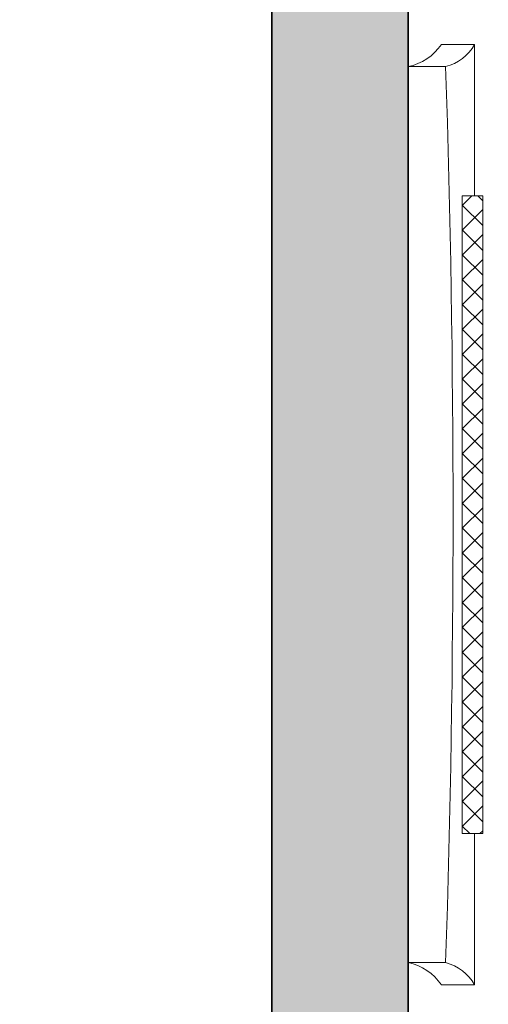
# Model space of a CAD drawing. Units: inches. Extents: x 2083 to 3317, y 1141 to 2115.
# Tile 4 of 256: x 2210 to 2241, y 1296 to 1361. Entities that reach past the tile are written whole.
import ezdxf

# ---------------------------------------------------------------- set-up
doc = ezdxf.new("R2010")
doc.units = ezdxf.units.IN
for name, color, linetype, lineweight in [('A-ANNO-DIMS', 2, 'Continuous', 18), ('A-FURN', 8, 'Continuous', 18), ('A-WALL', 7, 'Continuous', 35), ('www.cadblocksfree.com', 7, 'Continuous', 9)]:
    doc.layers.add(name, color=color, linetype=linetype, lineweight=lineweight)
doc.layers.add('A-WALL-PATT', color=251, linetype='Continuous', lineweight=13, true_color=0x636466)
doc.styles.get("Standard").update_dxf_attribs({"font": 'arial.ttf'})
doc.dimstyles.new('ISO-25', dxfattribs={"dimtxt": 12, "dimasz": 12, "dimexe": 1.25, "dimexo": 0.625, "dimtad": 1, "dimlunit": 3, "dimtxsty": 'Standard', "dimcen": 2.5, "dimadec": 0, "dimazin": 0, "dimtfac": 1, "dimtmove": 0, "dimatfit": 3, "dimfxl": 1, "dimarcsym": 0})

# ---------------------------------------------------------------- blocks, each defined once
blk = doc.blocks.new('bed')
at = {"layer": 'www.cadblocksfree.com', "ltscale": 0.2}
h = blk.add_hatch(dxfattribs=at)
h.set_pattern_fill('ANSI37,_O', color=256, scale=0.393701)
h.set_pattern_definition([(45, (2420.7222, -262.9689), (-0.8838835, 0.8838835), []), (135, (2420.7222, -262.9689), (-0.8838835, -0.8838835), [])])
h.paths.add_polyline_path([(3417.573, 1472.402), (3372.192, 1472.402), (3372.192, 1470.941), (3417.573, 1470.941)])
for p, q in [((3363.002, 1473.586), (3363.002, 1476.249)), ((3426.763, 1473.586), (3426.763, 1476.249)), ((3372.192, 1472.402), (3417.573, 1472.402)), ((3372.192, 1470.941), (3372.192, 1472.402)), ((3417.573, 1470.941), (3417.573, 1472.402)), ((3372.192, 1470.941), (3417.573, 1470.941))]:
    blk.add_line(p, q, dxfattribs=at)
for points in [[(3426.763, 1476.249), (3363.002, 1476.249)], [(3361.418, 1473.886), (3361.418, 1471.524), (3372.192, 1471.524)], [(3417.573, 1471.524), (3428.347, 1471.524), (3428.347, 1473.886)]]:
    blk.add_lwpolyline(points, dxfattribs=at)
for centre, radius, start, end in [((3359.334, 1476.997), 3.744, 303.82711, 348.4775), ((3430.432, 1476.997), 3.744, 191.5225, 236.17289), ((3359.844, 1474.373), 3.255, 298.91758, 345.9939), ((3394.883, 2431.358), 958.303, 268.093559, 271.906441), ((3429.921, 1474.373), 3.255, 194.0061, 241.08242)]:
    blk.add_arc(centre, radius, start, end, dxfattribs=at)
blk = doc.blocks.new('*D13')
at = {"layer": 'A-ANNO-DIMS', "color": 0, "lineweight": -2, "transparency": 16777216}
for p, q in [((2226.335, 1477.761), (2191.976, 1477.761)), ((2193.226, 1465.761), (2193.226, 1275.261)), ((2226.335, 1263.261), (2191.976, 1263.261))]:
    blk.add_line(p, q, dxfattribs=at)
at = {"layer": 'A-ANNO-DIMS', "color": 0, "transparency": 16777216}
for points in [[(2191.226, 1465.761), (2195.226, 1465.761), (2193.226, 1477.761)], [(2191.226, 1275.261), (2195.226, 1275.261), (2193.226, 1263.261)]]:
    blk.add_solid(points, dxfattribs=at)
at = {"layer": 'Defpoints', "color": 0, "transparency": 16777216}
for p in [(2226.96, 1477.761), (2193.226, 1263.261), (2226.96, 1263.261)]:
    blk.add_point(p, dxfattribs=at)
at = {"layer": 'A-ANNO-DIMS', "color": 0, "transparency": 16777216, "insert": (2186.474, 1370.511), "char_height": 12, "attachment_point": 5, "rotation": 90}
blk.add_mtext('17\'-10.5"', dxfattribs=at)
blk = doc.blocks.new('*D22')
at = {"layer": 'A-ANNO-DIMS', "color": 0, "lineweight": -2, "transparency": 16777216}
for p, q in [((2235.96, 1362.739), (2235.96, 1376.309)), ((2322.26, 1362.739), (2322.26, 1376.309)), ((2235.96, 1375.059), (2083.007, 1375.059)), ((2310.26, 1375.059), (2247.96, 1375.059))]:
    blk.add_line(p, q, dxfattribs=at)
at = {"layer": 'A-ANNO-DIMS', "color": 0, "transparency": 16777216}
for points in [[(2247.96, 1377.059), (2247.96, 1373.059), (2235.96, 1375.059)], [(2310.26, 1377.059), (2310.26, 1373.059), (2322.26, 1375.059)]]:
    blk.add_solid(points, dxfattribs=at)
at = {"layer": 'Defpoints', "color": 0, "transparency": 16777216}
for p in [(2235.96, 1375.059), (2235.96, 1362.114), (2322.26, 1362.114)]:
    blk.add_point(p, dxfattribs=at)
at = {"layer": 'A-ANNO-DIMS', "color": 0, "transparency": 16777216, "insert": (2153.483, 1381.889), "char_height": 12, "attachment_point": 5}
blk.add_mtext('BED 7\'-2 1/2" TYP.', dxfattribs=at)
blk = doc.blocks.new('*D47')
at = {"layer": 'A-ANNO-DIMS', "color": 0, "lineweight": -2, "transparency": 16777216}
for p, q in [((2235.335, 1416.261), (2173.36, 1416.261)), ((2174.61, 1284.261), (2174.61, 1404.261)), ((2235.335, 1272.261), (2173.36, 1272.261))]:
    blk.add_line(p, q, dxfattribs=at)
at = {"layer": 'A-ANNO-DIMS', "color": 0, "transparency": 16777216}
for points in [[(2172.61, 1404.261), (2176.61, 1404.261), (2174.61, 1416.261)], [(2172.61, 1284.261), (2176.61, 1284.261), (2174.61, 1272.261)]]:
    blk.add_solid(points, dxfattribs=at)
at = {"layer": 'Defpoints', "color": 0, "transparency": 16777216}
for p in [(2174.61, 1416.261), (2235.96, 1416.261), (2235.96, 1272.261)]:
    blk.add_point(p, dxfattribs=at)
at = {"layer": 'A-ANNO-DIMS', "color": 0, "transparency": 16777216, "insert": (2167.858, 1344.261), "char_height": 12, "attachment_point": 5, "rotation": 90}
blk.add_mtext('12\'-0"', dxfattribs=at)

msp = doc.modelspace()

# ---------------------------------------------------------------- hatches: boundary and pattern name
at = {"layer": 'A-WALL-PATT'}
h = msp.add_hatch(color=256, dxfattribs=at)
h.dxf.hatch_style = 1
h.paths.add_polyline_path([(3126.96, 2020.761), (2748.96, 2020.761), (2604.96, 2020.761), (2226.96, 2020.761), (2226.96, 1702.761), (2466.96, 1702.761), (2466.96, 1582.761), (2418.96, 1582.761), (2418.96, 1477.761), (2226.96, 1477.761), (2226.96, 1263.261), (2544.96, 1263.261), (2544.96, 1411.761), (2604.96, 1411.761), (2685.96, 1411.761), (2685.96, 1420.761), (2604.96, 1420.761), (2604.96, 1573.761), (2604.96, 1702.761), (2604.96, 2011.761), (2748.96, 2011.761), (2748.96, 1702.761), (2862.96, 1702.761), (2862.96, 1621.761), (2871.96, 1621.761), (2871.96, 1702.761), (2883.96, 1702.761), (2883.96, 1706.939, -0.026459), (2883.96, 1711.761), (2757.96, 1711.761), (2757.96, 1807.761), (2787.96, 1807.761), (2787.96, 1812.261), (2757.96, 1812.261), (2757.96, 2011.761), (2877.96, 2011.761), (2877.96, 1812.261), (2847.96, 1812.261), (2847.96, 1807.761), (2889.836, 1807.761), (2889.836, 1812.261), (2882.46, 1812.261), (2882.46, 2011.761), (3117.96, 2011.761), (3117.96, 1812.261), (2937.836, 1812.261), (2937.836, 1807.761), (2995.71, 1807.761), (2995.71, 1796.118), (3000.21, 1796.118), (3000.21, 1807.761), (3117.96, 1807.761), (3117.96, 1711.761), (3000.21, 1711.761), (3000.21, 1760.118), (2998.573, 1760.118, -0.020711), (2995.71, 1760.118), (2995.71, 1711.761), (2931.96, 1711.761), (2931.96, 1702.761), (3126.96, 1702.761)])
h.paths.add_polyline_path([(2471.46, 2011.761), (2471.46, 1810.011), (2462.717, 1810.011), (2462.717, 1805.511), (2505.96, 1805.511), (2505.96, 1810.011), (2475.96, 1810.011), (2475.96, 2011.761), (2595.96, 2011.761), (2595.96, 1810.011), (2565.96, 1810.011), (2565.96, 1805.511), (2595.96, 1805.511), (2595.96, 1711.761), (2235.96, 1711.761), (2235.96, 1805.511), (2353.71, 1805.511), (2353.71, 1796.054), (2358.21, 1796.054), (2358.21, 1805.511), (2414.717, 1805.511), (2414.717, 1810.011), (2235.96, 1810.011), (2235.96, 2011.761)], flags=16)
h.paths.add_polyline_path([(2270.205, 1994.61), (2270.205, 1970.61), (2246.205, 1970.61), (2246.205, 1994.61)], flags=0)
edge = h.paths.add_edge_path(flags=0)
edge.add_ellipse((2332.027, 1899.798), major_axis=(-3.043, 3.043), ratio=0.168252, start_angle=-161.33217, end_angle=-156.30711, ccw=False)
edge.add_ellipse((2333.082, 1898.744), major_axis=(-1.055, 1.055), ratio=0.453532, start_angle=-123.37102, end_angle=-94.15911)
edge = h.paths.add_edge_path(flags=0)
edge.add_ellipse((2332.027, 1968.876), major_axis=(3.043, 3.043), ratio=0.168252, start_angle=18.66783, end_angle=23.69289)
edge.add_spline(control_points=[(2332.926, 1970.691), (2332.227, 1970.336), (2330.894, 1969.659), (2328.413, 1970.932), (2327.204, 1967.749), (2324.71, 1969.956), (2322.533, 1967.012), (2320.013, 1971.296), (2317.68, 1968.158), (2316.041, 1967.102), (2315.427, 1966.81)], knot_values=[0, 0, 0, 0, 2.267059, 4.324559, 6.685584, 8.878641, 11.121502, 14.300359, 17.755284, 19.732645, 19.732645, 19.732645, 19.732645], degree=3, periodic=0)
edge.add_ellipse((2332.027, 1968.876), major_axis=(3.043, 3.043), ratio=0.168252, start_angle=18.66783, end_angle=23.69289, ccw=False)
edge.add_ellipse((2333.082, 1969.931), major_axis=(1.055, 1.055), ratio=0.453532, start_angle=56.62898, end_angle=85.84089, ccw=False)
edge = h.paths.add_edge_path(flags=0)
edge.add_spline(control_points=[(2296.428, 1967.988), (2293.628, 1965.336), (2287.704, 1959.727), (2299.744, 1949.996), (2294.533, 1935.669), (2290.573, 1920.604), (2293.394, 1909.974), (2296.185, 1904.967)], knot_values=[0.099185, 0.099185, 0.099185, 0.099185, 0.345301, 0.619822, 0.982653, 1.386093, 1.810555, 1.810555, 1.810555, 1.810555], degree=3, periodic=0)
edge.add_spline(control_points=[(2296.185, 1904.967), (2297.384, 1902.619), (2298.001, 1901.949), (2298.553, 1901.468)], knot_values=[0.006246, 0.006246, 0.006246, 0.006246, 0.055476, 0.055476, 0.055476, 0.055476], degree=3, periodic=0)
edge.add_spline(control_points=[(2298.553, 1901.468), (2297.259, 1900.923), (2295.225, 1900.232), (2293.06, 1900.614), (2292.101, 1900.788), (2292.09, 1900.791)], knot_values=[0.312835, 0.312835, 0.312835, 0.312835, 0.40178, 0.474987, 0.475903, 0.475903, 0.475903, 0.475903], degree=3, periodic=0)
edge.add_arc((2292.794, 1904.664), 3.937, 215.4209, 259.69818, ccw=False)
edge.add_spline(control_points=[(2289.585, 1902.382), (2289.477, 1902.535), (2289.368, 1902.688), (2289.261, 1902.841)], knot_values=[0.102872, 0.102872, 0.102872, 0.102872, 0.116896, 0.116896, 0.116896, 0.116896], degree=3, periodic=0)
edge.add_spline(control_points=[(2289.261, 1902.841), (2288.687, 1902.55), (2287.64, 1902.02), (2285.881, 1901.874), (2283.853, 1901.504), (2281.72, 1899.711), (2278.467, 1899.493), (2276.157, 1901.883), (2272.259, 1899.804), (2267.778, 1901.843), (2262.244, 1900.184), (2257.415, 1901.782), (2254.318, 1900.726), (2253.178, 1900.337)], knot_values=[0, 0, 0, 0, 1.907977, 3.477176, 5.261074, 7.972851, 11.680248, 13.717921, 16.939592, 22.789562, 27.502503, 33.595215, 37.145618, 37.145618, 37.145618, 37.145618], degree=3, periodic=0)
edge.add_line((2253.178, 1900.337), (2250.244, 1902.841))
edge.add_line((2250.244, 1902.841), (2250.244, 1965.833))
edge.add_line((2250.244, 1965.833), (2253.178, 1968.337))
edge.add_spline(control_points=[(2253.178, 1968.337), (2254.318, 1967.948), (2257.415, 1966.892), (2262.244, 1968.49), (2267.778, 1966.831), (2271.527, 1968.537), (2273.876, 1967.828), (2274.207, 1967.728)], knot_values=[0, 0, 0, 0, 0.09018, 0.244935, 0.364644, 0.513233, 0.537855, 0.537855, 0.537855, 0.537855], degree=3, periodic=0)
edge.add_arc((2274.353, 1963.793), 3.937, 72.05113, 92.12795, ccw=False)
edge.add_arc((2281.297, 1985.23), 18.596, 252.05113, 288.56572)
edge.add_arc((2292.317, 1956.029), 12.646, 71.02679, 113.77822, ccw=False)
edge = h.paths.add_edge_path(flags=0)
edge.add_spline(control_points=[(2274.899, 1951.856), (2275.066, 1951.617), (2275.233, 1951.377), (2275.398, 1951.136)], knot_values=[1.409916, 1.409916, 1.409916, 1.409916, 1.43159, 1.43159, 1.43159, 1.43159], degree=3, periodic=0)
edge.add_spline(control_points=[(2275.398, 1951.136), (2275.792, 1950.562), (2276.179, 1949.984), (2276.546, 1949.397)], knot_values=[1.358238, 1.358238, 1.358238, 1.358238, 1.409916, 1.409916, 1.409916, 1.409916], degree=3, periodic=0)
edge.add_line((2276.546, 1949.397), (2277.437, 1947.862))
edge.add_spline(control_points=[(2277.437, 1947.862), (2276.304, 1945.673), (2274.64, 1942.427), (2274.632, 1938.094), (2272.799, 1930.852), (2274.356, 1943.897), (2275.948, 1947.923), (2276.546, 1949.397)], knot_values=[0.005632, 0.005632, 0.005632, 0.005632, 0.186014, 0.266002, 0.357087, 0.59639, 0.739732, 0.739732, 0.739732, 0.739732], degree=3, periodic=0)
edge.add_spline(control_points=[(2276.546, 1949.397), (2276.179, 1949.984), (2275.792, 1950.562), (2275.398, 1951.136)], knot_values=[1.358238, 1.358238, 1.358238, 1.358238, 1.409916, 1.409916, 1.409916, 1.409916], degree=3, periodic=0)
edge.add_spline(control_points=[(2275.398, 1951.136), (2274.943, 1950.08), (2274.208, 1948.025), (2273.935, 1944.851), (2272.469, 1937.627), (2273.466, 1945.696), (2274.701, 1951.059), (2274.899, 1951.856)], knot_values=[0.104364, 0.104364, 0.104364, 0.104364, 0.189636, 0.269624, 0.36071, 0.600013, 0.644622, 0.644622, 0.644622, 0.644622], degree=3, periodic=0)
h.paths.add_polyline_path([(2269.168, 1963.128, -0.357527), (2268.171, 1960.976, -0.092561), (2268.171, 1939.436, -0.357527), (2269.168, 1937.285, -0.357527), (2267.016, 1938.282, -0.164785), (2254.686, 1938.282, -0.357527), (2252.534, 1937.285, -0.357527), (2253.531, 1939.436, -0.092561), (2253.531, 1960.976, -0.357527), (2252.534, 1963.128, -0.357527), (2254.686, 1962.131, -0.164785), (2267.016, 1962.131, -0.357527)], flags=0)
h.paths.add_polyline_path([(2248.874, 1967.802), (2248.874, 1957.028), (2249.458, 1957.028), (2249.458, 1911.647), (2248.874, 1911.647), (2248.874, 1900.873), (2246.512, 1900.873, 0.197327), (2244.15, 1902.457), (2244.15, 1966.218, 0.197327), (2246.512, 1967.802)], flags=0)
h.paths.add_polyline_path([(2269.168, 1931.389, -0.357527), (2268.171, 1929.238, -0.092561), (2268.171, 1907.698, -0.357527), (2269.168, 1905.547, -0.357527), (2267.016, 1906.544, -0.164785), (2254.686, 1906.544, -0.357527), (2252.534, 1905.547, -0.357527), (2253.531, 1907.698, -0.092561), (2253.531, 1929.238, -0.357527), (2252.534, 1931.389, -0.357527), (2254.686, 1930.392, -0.164785), (2267.016, 1930.392, -0.357527)], flags=0)
edge = h.paths.add_edge_path(flags=0)
edge.add_spline(control_points=[(2276.197, 1906.724), (2276.168, 1909.029), (2276.114, 1913.372), (2270.598, 1924.925), (2273.905, 1919.013), (2275.922, 1916.262), (2275.475, 1912.402), (2277.258, 1910.381), (2276.696, 1908.225), (2276.646, 1906.813), (2276.618, 1906.008)], knot_values=[0, 0, 0, 0, 8.61026, 16.221274, 18.843057, 23.804898, 27.440828, 29.356102, 31.203478, 33.650687, 33.650687, 33.650687, 33.650687], degree=3, periodic=0)
edge.add_spline(control_points=[(2276.618, 1906.008), (2276.623, 1905.624), (2276.498, 1904.629), (2275.442, 1903.855), (2274.937, 1903.08), (2274.859, 1902.841)], knot_values=[0.156488, 0.156488, 0.156488, 0.156488, 0.184398, 0.231376, 0.250598, 0.250598, 0.250598, 0.250598], degree=3, periodic=0)
edge.add_line((2274.859, 1902.841), (2276.506, 1902.841))
edge.add_spline(control_points=[(2276.506, 1902.841), (2276.788, 1903.085), (2277.665, 1904.125), (2278.25, 1904.341), (2277.654, 1908.527), (2278.156, 1906.228), (2278.1, 1905.286), (2278.847, 1904.069), (2277.857, 1903.415), (2277.874, 1902.991), (2277.904, 1902.841)], knot_values=[0.059574, 0.059574, 0.059574, 0.059574, 0.080753, 0.103741, 0.16972, 0.176036, 0.207137, 0.240474, 0.262341, 0.27366, 0.27366, 0.27366, 0.27366], degree=3, periodic=0)
edge.add_line((2277.904, 1902.841), (2280.03, 1902.841))
edge.add_spline(control_points=[(2280.03, 1902.841), (2279.888, 1903.088), (2279.499, 1903.982), (2280.152, 1905.939), (2278.104, 1909.658), (2279.762, 1907.185), (2280.328, 1904.875), (2280.485, 1903.49), (2281.463, 1903.249), (2281.758, 1902.936), (2281.834, 1902.841)], knot_values=[0.013856, 0.013856, 0.013856, 0.013856, 0.034874, 0.088867, 0.107879, 0.126738, 0.158714, 0.193757, 0.217487, 0.226722, 0.226722, 0.226722, 0.226722], degree=3, periodic=0)
edge.add_spline(control_points=[(2281.834, 1902.841), (2281.788, 1902.827), (2281.647, 1902.783), (2281.396, 1902.859), (2281.088, 1902.985), (2280.721, 1903.061), (2280.333, 1903.026), (2280.125, 1902.899), (2280.03, 1902.841)], knot_values=[0, 0, 0, 0, 0.14413, 0.435517, 0.749276, 1.153046, 1.548371, 1.878348, 1.878348, 1.878348, 1.878348], degree=3, periodic=0)
edge.add_line((2280.03, 1902.841), (2277.904, 1902.841))
edge.add_spline(control_points=[(2277.904, 1902.841), (2277.893, 1902.796), (2277.865, 1902.68), (2277.607, 1902.687), (2277.274, 1902.801), (2276.838, 1902.62), (2276.584, 1902.789), (2276.506, 1902.841)], knot_values=[0, 0, 0, 0, 0.127189, 0.326199, 0.628009, 1.24357, 1.515331, 1.515331, 1.515331, 1.515331], degree=3, periodic=0)
edge.add_line((2276.506, 1902.841), (2274.859, 1902.841))
edge.add_spline(control_points=[(2274.859, 1902.841), (2274.814, 1902.899), (2274.725, 1903.013), (2274.493, 1903.119), (2274.244, 1902.961), (2273.937, 1903.185), (2273.614, 1902.983), (2273.408, 1902.883), (2273.322, 1902.841)], knot_values=[0, 0, 0, 0, 0.21843, 0.436957, 0.687977, 0.990379, 1.398396, 1.69185, 1.69185, 1.69185, 1.69185], degree=3, periodic=0)
edge.add_spline(control_points=[(2273.322, 1902.841), (2273.617, 1903.446), (2274.274, 1904.538), (2276.027, 1904.574), (2276.207, 1906.584), (2276.197, 1906.724)], knot_values=[0.012227, 0.012227, 0.012227, 0.012227, 0.059472, 0.106218, 0.134458, 0.134458, 0.134458, 0.134458], degree=3, periodic=0)
h.paths.add_polyline_path([(2270.776, 1897.79), (2270.776, 1873.79), (2246.776, 1873.79), (2246.776, 1897.79)], flags=0)
h.paths.add_polyline_path([(2353.71, 1760.005), (2353.71, 1760.054), (2358.21, 1760.054, -0.033729)], flags=0)
h.paths.add_polyline_path([(2321.819, 1737.529), (2341.995, 1737.529, -0.414214), (2343.203, 1736.321), (2343.203, 1721.021, -0.414214), (2341.995, 1719.813), (2321.819, 1719.813, -0.414214), (2320.611, 1721.021), (2320.611, 1736.321, -0.414214)], flags=0)
h.paths.add_polyline_path([(2324.235, 1736.321), (2339.579, 1736.321, -0.414214), (2341.995, 1733.905), (2341.995, 1725.45, -0.414214), (2339.579, 1723.034), (2333.681, 1723.034), (2333.845, 1722.045, -0.870646), (2335.425, 1721.826, -0.767327), (2333.923, 1721.423), (2331.291, 1721.423, -0.767327), (2329.788, 1721.826, -0.870646), (2331.368, 1722.045), (2331.533, 1723.034), (2324.235, 1723.034, -0.414214), (2321.819, 1725.45), (2321.819, 1733.905, -0.414214)], flags=0)
h.paths.add_polyline_path([(2570.484, 1928.615), (2589.684, 1928.615), (2590.169, 1928.615), (2590.169, 1904.993), (2570.484, 1904.993)], flags=0)
h.paths.add_polyline_path([(2574.447, 1927.264, -1), (2572.829, 1927.264, -1)], flags=0)
h.paths.add_polyline_path([(2573.09, 1926.941), (2573.925, 1927.776), (2574.148, 1927.553), (2573.313, 1926.718)], flags=0)
h.paths.add_polyline_path([(2578.779, 1919.73, -1), (2571.592, 1919.73, -1)], flags=0)
h.paths.add_polyline_path([(2578.385, 1919.73, -1), (2571.985, 1919.73, -1)], flags=0)
h.paths.add_polyline_path([(2331.596, 1729.476, -1), (2333.618, 1729.476, -1)], flags=0)
h.paths.add_polyline_path([(2578.034, 1927.264, -1), (2576.416, 1927.264, -1)], flags=0)
h.paths.add_polyline_path([(2576.689, 1927.531), (2576.912, 1927.754), (2577.747, 1926.919), (2577.524, 1926.696)], flags=0)
h.paths.add_polyline_path([(2578.139, 1909.86, -1), (2572.232, 1909.86, -1)], flags=0)
h.paths.add_polyline_path([(2577.745, 1909.86, -1), (2572.625, 1909.86, -1)], flags=0)
h.paths.add_polyline_path([(2583.798, 1927.264, -1), (2582.179, 1927.264, -1)], flags=0)
h.paths.add_polyline_path([(2582.719, 1927.754), (2583.554, 1926.919), (2583.331, 1926.696), (2582.496, 1927.531)], flags=0)
h.paths.add_polyline_path([(2582.496, 1927.531), (2582.719, 1927.754), (2583.554, 1926.919), (2583.331, 1926.696)], flags=0)
h.paths.add_polyline_path([(2587.739, 1920.53, -1), (2581.832, 1920.53, -1)], flags=0)
h.paths.add_polyline_path([(2587.345, 1920.53, -1), (2582.225, 1920.53, -1)], flags=0)
h.paths.add_polyline_path([(2587.385, 1927.264, -1), (2585.766, 1927.264, -1)], flags=0)
h.paths.add_polyline_path([(2586.082, 1926.98), (2586.917, 1927.815), (2587.14, 1927.593), (2586.305, 1926.758)], flags=0)
h.paths.add_polyline_path([(2588.379, 1910.66, -1), (2581.192, 1910.66, -1)], flags=0)
h.paths.add_polyline_path([(2587.985, 1910.66, -1), (2581.585, 1910.66, -1)], flags=0)
h.paths.add_polyline_path([(2417.168, 1729.478), (2437.344, 1729.478, -0.414214), (2438.552, 1728.27), (2438.552, 1712.969, -0.414214), (2437.344, 1711.761), (2417.168, 1711.761, -0.414214), (2415.96, 1712.969), (2415.96, 1728.27, -0.414214)], flags=0)
h.paths.add_polyline_path([(2419.584, 1728.27), (2434.928, 1728.27, -0.414214), (2437.344, 1725.854), (2437.344, 1717.398, -0.414214), (2434.928, 1714.983), (2429.029, 1714.983), (2429.194, 1713.994, -0.870646), (2430.774, 1713.775, -0.767327), (2429.271, 1713.372), (2426.64, 1713.372, -0.767327), (2425.137, 1713.775, -0.870646), (2426.717, 1713.994), (2426.882, 1714.983), (2419.584, 1714.983, -0.414214), (2417.168, 1717.398), (2417.168, 1725.854, -0.414214)], flags=0)
h.paths.add_polyline_path([(2419.584, 1728.27), (2434.928, 1728.27, -0.414214), (2437.344, 1725.854), (2437.344, 1717.398, -0.414214), (2434.928, 1714.983), (2429.029, 1714.983), (2428.358, 1719.009), (2427.553, 1719.009), (2426.882, 1714.983), (2419.584, 1714.983, -0.414214), (2417.168, 1717.398), (2417.168, 1725.854, -0.414214)], flags=0)
h.paths.add_polyline_path([(2426.944, 1721.425, -1), (2428.967, 1721.425, -1)], flags=0)
h.paths.add_polyline_path([(2475.96, 1702.761), (2595.96, 1702.761), (2595.96, 1582.761), (2475.96, 1582.761)], flags=16)
h.paths.add_polyline_path([(2427.96, 1573.761), (2595.96, 1573.761), (2595.96, 1468.761), (2595.96, 1420.761), (2384.46, 1420.761), (2384.46, 1468.761), (2427.96, 1468.761)], flags=16)
h.paths.add_polyline_path([(2379.96, 1468.761), (2379.96, 1420.761), (2235.96, 1420.761), (2235.96, 1468.761)], flags=16)
h.paths.add_polyline_path([(2317.816, 1466.696), (2337.992, 1466.696, -0.414214), (2339.2, 1465.488), (2339.2, 1450.187, -0.414214), (2337.992, 1448.979), (2317.816, 1448.979, -0.414214), (2316.608, 1450.187), (2316.608, 1465.488, -0.414214)], flags=0)
h.paths.add_polyline_path([(2320.232, 1465.488), (2335.576, 1465.488, -0.414214), (2337.992, 1463.072), (2337.992, 1454.616, -0.414214), (2335.576, 1452.2), (2329.677, 1452.2), (2329.842, 1451.212, -0.870646), (2331.422, 1450.992, -0.767327), (2329.92, 1450.59), (2327.288, 1450.59, -0.767327), (2325.785, 1450.992, -0.870646), (2327.365, 1451.212), (2327.53, 1452.2), (2320.232, 1452.2, -0.414214), (2317.816, 1454.616), (2317.816, 1463.072, -0.414214)], flags=0)
h.paths.add_polyline_path([(2320.232, 1465.488), (2335.576, 1465.488, -0.414214), (2337.992, 1463.072), (2337.992, 1454.616, -0.414214), (2335.576, 1452.2), (2329.677, 1452.2), (2329.006, 1456.227), (2328.201, 1456.227), (2327.53, 1452.2), (2320.232, 1452.2, -0.414214), (2317.816, 1454.616), (2317.816, 1463.072, -0.414214)], flags=0)
h.paths.add_polyline_path([(2327.593, 1458.643, -1), (2329.615, 1458.643, -1)], flags=0)
h.paths.add_polyline_path([(2244.412, 1433.34), (2241.921, 1433.34, -0.414214), (2240.018, 1435.244), (2240.018, 1440.953, -0.414211), (2241.921, 1442.856), (2244.412, 1442.856, -1.976472)], flags=0)
h.paths.add_polyline_path([(2245.357, 1434.398, -0.414214), (2245.357, 1441.799, -2.144098)], flags=0)
h.paths.add_polyline_path([(2535.96, 1416.261), (2535.96, 1272.261), (2235.96, 1272.261), (2235.96, 1416.261)], flags=16)
h.paths.add_polyline_path([(2260.12, 1384.293), (2260.12, 1362.039), (2237.865, 1362.039), (2237.865, 1384.293)], flags=0)
edge = h.paths.add_edge_path(flags=0)
edge.add_line((2318.252, 1362.093), (2318.146, 1362.001))
edge.add_ellipse((2317.445, 1360.431), major_axis=(2.822, 2.822), ratio=0.168252, start_angle=18.66783, end_angle=20.94813, ccw=False)
edge.add_ellipse((2318.423, 1361.409), major_axis=(0.978, 0.978), ratio=0.453532, start_angle=56.62898, end_angle=70.2262, ccw=False)
edge = h.paths.add_edge_path(flags=0)
edge.add_line((2319.107, 1295.571), (2319.015, 1295.677))
edge.add_ellipse((2317.445, 1296.378), major_axis=(-2.822, 2.822), ratio=0.168252, start_angle=-161.33217, end_angle=-159.05187, ccw=False)
edge.add_ellipse((2318.423, 1295.4), major_axis=(-0.978, 0.978), ratio=0.453532, start_angle=-123.37102, end_angle=-109.7738)
edge = h.paths.add_edge_path(flags=0)
edge.add_spline(control_points=[(2284.21, 1301.17), (2284.581, 1300.445), (2284.891, 1299.892), (2285.16, 1299.461)], knot_values=[0.039066, 0.039066, 0.039066, 0.039066, 0.055476, 0.055476, 0.055476, 0.055476], degree=3, periodic=0)
edge.add_line((2285.16, 1299.461), (2284.21, 1301.17))
edge = h.paths.add_edge_path(flags=0)
edge.add_line((2280.412, 1297.298), (2283.37, 1297.036))
edge.add_line((2283.37, 1297.036), (2286.406, 1297.926))
edge.add_spline(control_points=[(2286.406, 1297.926), (2285.305, 1297.463), (2284.345, 1297.129), (2283.37, 1297.036)], knot_values=[0.394369, 0.394369, 0.394369, 0.394369, 0.475903, 0.475903, 0.475903, 0.475903], degree=3, periodic=0)
edge.add_spline(control_points=[(2283.37, 1297.036), (2283.281, 1297.028), (2282.316, 1296.957), (2281.313, 1297.134), (2280.423, 1297.296), (2280.412, 1297.298)], knot_values=[0.312835, 0.312835, 0.312835, 0.312835, 0.320246, 0.393453, 0.394369, 0.394369, 0.394369, 0.394369], degree=3, periodic=0)
edge = h.paths.add_edge_path(flags=0)
edge.add_line((2284.436, 1359.607), (2280.446, 1355.328))
edge.add_line((2280.446, 1355.328), (2279.58, 1351.018))
edge.add_line((2279.58, 1351.018), (2282.413, 1346.58))
edge.add_spline(control_points=[(2282.413, 1346.58), (2283.153, 1345.589), (2284.253, 1344.029), (2284.801, 1342.387), (2284.935, 1341.806)], knot_values=[1.240098, 1.240098, 1.240098, 1.240098, 1.332892, 1.382712, 1.382712, 1.382712, 1.382712], degree=3, periodic=0)
edge.add_spline(control_points=[(2284.935, 1341.806), (2285.319, 1340.141), (2285.233, 1338.409), (2284.91, 1336.654)], knot_values=[1.097484, 1.097484, 1.097484, 1.097484, 1.240098, 1.240098, 1.240098, 1.240098], degree=3, periodic=0)
edge.add_spline(control_points=[(2284.91, 1336.654), (2284.587, 1334.899), (2284.027, 1333.12), (2283.463, 1331.361)], knot_values=[0.95487, 0.95487, 0.95487, 0.95487, 1.097484, 1.097484, 1.097484, 1.097484], degree=3, periodic=0)
edge.add_line((2283.463, 1331.361), (2281.89, 1326.153))
edge.add_line((2281.89, 1326.153), (2280.756, 1321.056))
edge.add_line((2280.756, 1321.056), (2280.299, 1316.002))
edge.add_line((2280.299, 1316.002), (2280.716, 1310.95))
edge.add_line((2280.716, 1310.95), (2282.028, 1305.972))
edge.add_line((2282.028, 1305.972), (2284.21, 1301.17))
edge.add_spline(control_points=[(2284.21, 1301.17), (2283.341, 1302.73), (2282.612, 1304.336), (2282.028, 1305.972)], knot_values=[0.099185, 0.099185, 0.099185, 0.099185, 0.241799, 0.241799, 0.241799, 0.241799], degree=3, periodic=0)
edge.add_spline(control_points=[(2282.028, 1305.972), (2281.444, 1307.608), (2281.005, 1309.273), (2280.716, 1310.95)], knot_values=[0.241799, 0.241799, 0.241799, 0.241799, 0.384413, 0.384413, 0.384413, 0.384413], degree=3, periodic=0)
edge.add_spline(control_points=[(2280.716, 1310.95), (2280.433, 1312.588), (2280.289, 1314.277), (2280.299, 1315.962), (2280.299, 1316.002)], knot_values=[0.384413, 0.384413, 0.384413, 0.384413, 0.523647, 0.527028, 0.527028, 0.527028, 0.527028], degree=3, periodic=0)
edge.add_spline(control_points=[(2280.299, 1316.002), (2280.312, 1317.687), (2280.478, 1319.368), (2280.756, 1321.056)], knot_values=[0.527028, 0.527028, 0.527028, 0.527028, 0.669642, 0.669642, 0.669642, 0.669642], degree=3, periodic=0)
edge.add_spline(control_points=[(2280.756, 1321.056), (2281.035, 1322.744), (2281.426, 1324.44), (2281.89, 1326.153)], knot_values=[0.669642, 0.669642, 0.669642, 0.669642, 0.812256, 0.812256, 0.812256, 0.812256], degree=3, periodic=0)
edge.add_spline(control_points=[(2281.89, 1326.153), (2282.264, 1327.533), (2282.788, 1329.262), (2283.353, 1331.018), (2283.463, 1331.361)], knot_values=[0.812256, 0.812256, 0.812256, 0.812256, 0.927087, 0.95487, 0.95487, 0.95487, 0.95487], degree=3, periodic=0)
edge.add_line((2283.463, 1331.361), (2284.91, 1336.654))
edge.add_line((2284.91, 1336.654), (2284.935, 1341.806))
edge.add_line((2284.935, 1341.806), (2282.413, 1346.58))
edge.add_spline(control_points=[(2282.413, 1346.58), (2281.275, 1348.104), (2280.078, 1349.57), (2279.58, 1351.018)], knot_values=[1.382712, 1.382712, 1.382712, 1.382712, 1.525326, 1.525326, 1.525326, 1.525326], degree=3, periodic=0)
edge.add_spline(control_points=[(2279.58, 1351.018), (2279.443, 1351.415), (2279.136, 1352.857), (2279.735, 1354.29), (2280.446, 1355.328)], knot_values=[1.525326, 1.525326, 1.525326, 1.525326, 1.564439, 1.667941, 1.667941, 1.667941, 1.667941], degree=3, periodic=0)
edge.add_spline(control_points=[(2280.446, 1355.328), (2281.426, 1356.758), (2282.931, 1358.183), (2284.436, 1359.607)], knot_values=[1.667941, 1.667941, 1.667941, 1.667941, 1.810555, 1.810555, 1.810555, 1.810555], degree=3, periodic=0)
edge.add_arc((2280.623, 1348.518), 11.726, 71.02679, 113.77822)
edge.add_arc((2270.405, 1375.595), 17.244, 252.05113, 288.56572, ccw=False)
edge.add_arc((2263.966, 1355.718), 3.651, 72.05113, 92.12795)
edge.add_arc((2263.966, 1355.718), 3.651, 92.12795, 177.98513)
edge.add_spline(control_points=[(2260.318, 1355.846), (2260.26, 1354.221), (2260.551, 1350.187), (2262.999, 1346.766), (2264.473, 1344.649)], knot_values=[1.43159, 1.43159, 1.43159, 1.43159, 1.564144, 1.770695, 1.770695, 1.770695, 1.770695], degree=3, periodic=0)
edge.add_line((2264.473, 1344.649), (2264.936, 1343.983))
edge.add_spline(control_points=[(2263.801, 1340.248), (2263.843, 1340.514), (2264.067, 1341.756), (2264.513, 1343.002), (2264.935, 1343.981)], knot_values=[0.53657, 0.53657, 0.53657, 0.53657, 0.559349, 0.644622, 0.644622, 0.644622, 0.644622], degree=3, periodic=0)
edge.add_spline(control_points=[(2264.935, 1343.981), (2265.118, 1343.715), (2265.299, 1343.448), (2265.477, 1343.179)], knot_values=[1.384077, 1.384077, 1.384077, 1.384077, 1.409916, 1.409916, 1.409916, 1.409916], degree=3, periodic=0)
edge.add_spline(control_points=[(2265.477, 1343.179), (2265.655, 1342.911), (2265.829, 1342.641), (2265.999, 1342.369)], knot_values=[1.358238, 1.358238, 1.358238, 1.358238, 1.384077, 1.384077, 1.384077, 1.384077], degree=3, periodic=0)
edge.add_line((2265.999, 1342.369), (2266.826, 1340.946))
edge.add_spline(control_points=[(2266.826, 1340.946), (2268.894, 1337.09), (2271.398, 1325.843), (2270.516, 1310.569), (2275.919, 1301.861), (2277.79, 1299.199)], knot_values=[0.116896, 0.116896, 0.116896, 0.116896, 0.472987, 1.050969, 1.313793, 1.313793, 1.313793, 1.313793], degree=3, periodic=0)
edge.add_spline(control_points=[(2277.79, 1299.199), (2277.839, 1299.128), (2277.889, 1299.057), (2277.94, 1298.987)], knot_values=[0.109884, 0.109884, 0.109884, 0.109884, 0.116896, 0.116896, 0.116896, 0.116896], degree=3, periodic=0)
edge.add_line((2277.94, 1298.987), (2277.789, 1299.199))
edge.add_spline(control_points=[(2277.789, 1299.199), (2277.257, 1298.929), (2276.286, 1298.438), (2275.039, 1298.334), (2274.383, 1298.239), (2274.215, 1298.209)], knot_values=[33.12187, 33.12187, 33.12187, 33.12187, 35.029056, 36.598255, 37.144827, 37.144827, 37.144827, 37.144827], degree=3, periodic=0)
edge.add_line((2274.215, 1298.209), (2273.073, 1297.893))
edge.add_spline(control_points=[(2273.073, 1297.893), (2272.323, 1297.58), (2271.039, 1296.511), (2269.248, 1296.226), (2268.423, 1296.375)], knot_values=[26.532584, 26.532584, 26.532584, 26.532584, 29.198919, 31.839101, 31.839101, 31.839101, 31.839101], degree=3, periodic=0)
edge.add_line((2268.423, 1296.375), (2263.879, 1297.458))
edge.add_spline(control_points=[(2263.879, 1297.458), (2263.556, 1297.359), (2261.86, 1296.839), (2260.239, 1297.282), (2258.933, 1297.516)], knot_values=[15.919551, 15.919551, 15.919551, 15.919551, 16.939592, 21.226067, 21.226067, 21.226067, 21.226067], degree=3, periodic=0)
edge.add_line((2258.933, 1297.516), (2254.055, 1297.329))
edge.add_spline(control_points=[(2254.055, 1297.329), (2253.756, 1297.296), (2252.114, 1297.165), (2250.462, 1297.544), (2249.13, 1297.668)], knot_values=[5.306517, 5.306517, 5.306517, 5.306517, 6.276435, 10.613034, 10.613034, 10.613034, 10.613034], degree=3, periodic=0)
edge.add_line((2249.13, 1297.668), (2244.332, 1296.878))
edge.add_line((2244.332, 1296.878), (2241.611, 1299.199))
edge.add_line((2241.611, 1299.199), (2241.611, 1357.609))
edge.add_line((2241.611, 1357.609), (2244.332, 1359.931))
edge.add_line((2244.332, 1359.931), (2252.729, 1359.543))
edge.add_spline(control_points=[(2252.729, 1359.543), (2252.871, 1359.546), (2253.306, 1359.548), (2253.74, 1359.514), (2254.032, 1359.482)], knot_values=[0.233291, 0.233291, 0.233291, 0.233291, 0.244935, 0.268927, 0.268927, 0.268927, 0.268927], degree=3, periodic=0)
edge.add_line((2254.032, 1359.482), (2259.587, 1359.416))
edge.add_spline(control_points=[(2259.587, 1359.416), (2260.677, 1359.629), (2262.073, 1359.897), (2263.524, 1359.459), (2263.83, 1359.366)], knot_values=[0.422516, 0.422516, 0.422516, 0.422516, 0.513233, 0.537855, 0.537855, 0.537855, 0.537855], degree=3, periodic=0)
edge.add_arc((2263.966, 1355.718), 3.651, 72.05113, 92.12795, ccw=False)
edge.add_arc((2270.405, 1375.595), 17.244, 252.05113, 288.56572)
edge.add_arc((2280.623, 1348.518), 11.726, 71.02679, 113.77822, ccw=False)
h.paths.add_polyline_path([(2240.341, 1359.435), (2240.341, 1349.444), (2240.882, 1349.444), (2240.882, 1307.365), (2240.341, 1307.365), (2240.341, 1297.374), (2238.15, 1297.374, 0.197327), (2235.96, 1298.843), (2235.96, 1357.966, 0.197327), (2238.15, 1359.435)], flags=0)
h.paths.add_polyline_path([(2259.158, 1355.101, -0.357527), (2258.233, 1353.106, -0.092561), (2258.233, 1333.133, -0.357527), (2259.158, 1331.138, -0.357527), (2257.163, 1332.062, -0.164785), (2245.729, 1332.062, -0.357527), (2243.735, 1331.138, -0.357527), (2244.659, 1333.133, -0.092561), (2244.659, 1353.106, -0.357527), (2243.735, 1355.101, -0.357527), (2245.729, 1354.176, -0.164785), (2257.163, 1354.176, -0.357527)], flags=0)
edge = h.paths.add_edge_path(flags=0)
edge.add_line((2265.999, 1342.369), (2266.826, 1340.946))
edge.add_line((2266.826, 1340.946), (2265.308, 1337.814))
edge.add_line((2265.308, 1337.814), (2264.358, 1334.653))
edge.add_line((2264.358, 1334.653), (2264.262, 1333.8))
edge.add_spline(control_points=[(2264.262, 1333.8), (2264.208, 1333.187), (2264.162, 1332.366), (2264.007, 1331.414), (2263.969, 1331.202)], knot_values=[0.464444, 0.464444, 0.464444, 0.464444, 0.516691, 0.531608, 0.531608, 0.531608, 0.531608], degree=3, periodic=0)
edge.add_spline(control_points=[(2263.969, 1331.202), (2263.775, 1330.119), (2263.424, 1328.791), (2263.257, 1328.531), (2263.234, 1328.515)], knot_values=[0.372682, 0.372682, 0.372682, 0.372682, 0.44885, 0.464444, 0.464444, 0.464444, 0.464444], degree=3, periodic=0)
edge.add_spline(control_points=[(2263.234, 1328.515), (2263.096, 1328.42), (2263.131, 1329.301), (2263.275, 1330.616)], knot_values=[0.280919, 0.280919, 0.280919, 0.280919, 0.372682, 0.372682, 0.372682, 0.372682], degree=3, periodic=0)
edge.add_spline(control_points=[(2263.275, 1330.616), (2263.419, 1331.93), (2263.672, 1333.677), (2263.97, 1335.315)], knot_values=[0.189157, 0.189157, 0.189157, 0.189157, 0.280919, 0.280919, 0.280919, 0.280919], degree=3, periodic=0)
edge.add_spline(control_points=[(2263.97, 1335.315), (2264.1, 1336.032), (2264.419, 1337.622), (2264.755, 1338.864), (2264.947, 1339.491)], knot_values=[0.097394, 0.097394, 0.097394, 0.097394, 0.137578, 0.189157, 0.189157, 0.189157, 0.189157], degree=3, periodic=0)
edge.add_spline(control_points=[(2264.947, 1339.491), (2265.29, 1340.606), (2265.644, 1341.494), (2265.999, 1342.369)], knot_values=[0.005632, 0.005632, 0.005632, 0.005632, 0.097394, 0.097394, 0.097394, 0.097394], degree=3, periodic=0)
h.paths.add_polyline_path([(2259.158, 1325.671, -0.357527), (2258.233, 1323.676, -0.092561), (2258.233, 1303.703, -0.357527), (2259.158, 1301.708, -0.357527), (2257.163, 1302.633, -0.164785), (2245.729, 1302.633, -0.357527), (2243.735, 1301.708, -0.357527), (2244.659, 1303.703, -0.092561), (2244.659, 1323.676, -0.357527), (2243.735, 1325.671, -0.357527), (2245.729, 1324.747, -0.164785), (2257.163, 1324.747, -0.357527)], flags=0)
edge = h.paths.add_edge_path(flags=0)
edge.add_spline(control_points=[(2261.709, 1317.311), (2261.679, 1317.418), (2261.762, 1317.389), (2262.491, 1316.09), (2262.962, 1315.301)], knot_values=[14.955861, 14.955861, 14.955861, 14.955861, 16.221274, 18.694826, 18.694826, 18.694826, 18.694826], degree=3, periodic=0)
edge.add_spline(control_points=[(2262.962, 1315.301), (2262.99, 1315.254), (2263.702, 1314.067), (2264.349, 1313.127), (2264.73, 1312.164)], knot_values=[18.694826, 18.694826, 18.694826, 18.694826, 18.843057, 22.433791, 22.433791, 22.433791, 22.433791], degree=3, periodic=0)
edge.add_spline(control_points=[(2264.73, 1312.164), (2264.876, 1311.796), (2265.177, 1310.77), (2265.143, 1309.559), (2265.248, 1308.824)], knot_values=[22.433791, 22.433791, 22.433791, 22.433791, 23.804898, 26.172756, 26.172756, 26.172756, 26.172756], degree=3, periodic=0)
edge.add_line((2265.248, 1308.824), (2265.851, 1307.172))
edge.add_spline(control_points=[(2265.851, 1307.172), (2266.065, 1306.822), (2266.384, 1306.332), (2266.424, 1305.781), (2266.42, 1305.611)], knot_values=[28.062562, 28.062562, 28.062562, 28.062562, 29.356102, 29.911721, 29.911721, 29.911721, 29.911721], degree=3, periodic=0)
edge.add_spline(control_points=[(2266.42, 1305.611), (2266.416, 1305.433), (2266.394, 1305.25), (2266.365, 1305.066)], knot_values=[29.911721, 29.911721, 29.911721, 29.911721, 30.497837, 30.497837, 30.497837, 30.497837], degree=3, periodic=0)
edge.add_line((2266.365, 1305.066), (2266.066, 1302.136))
edge.add_spline(control_points=[(2266.066, 1302.136), (2266.071, 1301.78), (2265.998, 1301.2), (2265.663, 1300.759), (2265.509, 1300.586)], knot_values=[0.156488, 0.156488, 0.156488, 0.156488, 0.184398, 0.203543, 0.203543, 0.203543, 0.203543], degree=3, periodic=0)
edge.add_line((2265.509, 1300.586), (2264.435, 1299.199))
edge.add_line((2264.435, 1299.199), (2265.962, 1299.199))
edge.add_line((2265.962, 1299.199), (2267.336, 1301.175))
edge.add_line((2267.336, 1301.175), (2267.312, 1301.986))
edge.add_spline(control_points=[(2267.312, 1301.986), (2267.261, 1302.862), (2267.16, 1303.737), (2267.271, 1303.326)], knot_values=[0.126229, 0.126229, 0.126229, 0.126229, 0.166617, 0.166617, 0.166617, 0.166617], degree=3, periodic=0)
edge.add_spline(control_points=[(2267.271, 1303.326), (2267.28, 1303.294), (2267.31, 1303.175), (2267.373, 1302.884), (2267.406, 1302.683), (2267.418, 1302.601)], knot_values=[0.166617, 0.166617, 0.166617, 0.166617, 0.16972, 0.176036, 0.180765, 0.180765, 0.180765, 0.180765], degree=3, periodic=0)
edge.add_spline(control_points=[(2267.744, 1300.988), (2267.688, 1301.151), (2267.481, 1301.657), (2267.484, 1302.145), (2267.418, 1302.601)], knot_values=[0.180765, 0.180765, 0.180765, 0.180765, 0.193767, 0.220139, 0.220139, 0.220139, 0.220139], degree=3, periodic=0)
edge.add_line((2267.418, 1302.601), (2267.744, 1300.988))
edge.add_spline(control_points=[(2267.744, 1300.988), (2267.832, 1300.732), (2267.932, 1300.31), (2267.555, 1299.975), (2267.429, 1299.829)], knot_values=[0.220139, 0.220139, 0.220139, 0.220139, 0.240474, 0.25489, 0.25489, 0.25489, 0.25489], degree=3, periodic=0)
edge.add_line((2267.429, 1299.829), (2267.258, 1299.199))
edge.add_line((2267.258, 1299.199), (2269.23, 1299.199))
edge.add_spline(control_points=[(2269.23, 1299.199), (2269.099, 1299.429), (2268.843, 1300.016), (2269.012, 1300.916), (2268.947, 1301.661)], knot_values=[0.013856, 0.013856, 0.013856, 0.013856, 0.034874, 0.067073, 0.067073, 0.067073, 0.067073], degree=3, periodic=0)
edge.add_line((2268.947, 1301.661), (2268.432, 1303.603))
edge.add_spline(control_points=[(2268.432, 1303.603), (2268.176, 1304.192), (2267.596, 1305.251), (2268.041, 1304.623), (2268.251, 1304.282)], knot_values=[0.090155, 0.090155, 0.090155, 0.090155, 0.107879, 0.120289, 0.120289, 0.120289, 0.120289], degree=3, periodic=0)
edge.add_spline(control_points=[(2268.251, 1304.282), (2268.361, 1304.105), (2269.058, 1302.918), (2269.383, 1301.59), (2269.521, 1300.776), (2269.575, 1300.556)], knot_values=[0.120289, 0.120289, 0.120289, 0.120289, 0.126738, 0.158714, 0.173506, 0.173506, 0.173506, 0.173506], degree=3, periodic=0)
edge.add_line((2269.575, 1300.556), (2270.686, 1299.421))
edge.add_spline(control_points=[(2270.686, 1299.421), (2270.767, 1299.357), (2270.838, 1299.281), (2270.903, 1299.199)], knot_values=[0.21816, 0.21816, 0.21816, 0.21816, 0.226722, 0.226722, 0.226722, 0.226722], degree=3, periodic=0)
edge.add_line((2270.937, 1299.193), (2270.903, 1299.199))
edge.add_spline(control_points=[(2270.903, 1299.199), (2270.86, 1299.186), (2270.73, 1299.146), (2270.496, 1299.216), (2270.272, 1299.308), (2270.121, 1299.348), (2270.063, 1299.36)], knot_values=[0.939174, 0.939174, 0.939174, 0.939174, 1.083304, 1.374691, 1.68845, 1.878348, 1.878348, 1.878348, 1.878348], degree=3, periodic=0)
edge.add_line((2270.063, 1299.36), (2269.23, 1299.199))
edge.add_line((2269.23, 1299.199), (2267.258, 1299.199))
edge.add_spline(control_points=[(2267.258, 1299.199), (2267.248, 1299.157), (2267.223, 1299.05), (2266.984, 1299.057), (2266.809, 1299.116), (2266.677, 1299.109), (2266.637, 1299.105)], knot_values=[0.757665, 0.757665, 0.757665, 0.757665, 0.884854, 1.083864, 1.385675, 1.515331, 1.515331, 1.515331, 1.515331], degree=3, periodic=0)
edge.add_spline(control_points=[(2266.637, 1299.105), (2266.485, 1299.089), (2266.236, 1299.017), (2266.035, 1299.151), (2265.962, 1299.199)], knot_values=[0, 0, 0, 0, 0.485905, 0.757665, 0.757665, 0.757665, 0.757665], degree=3, periodic=0)
edge.add_line((2265.962, 1299.199), (2264.435, 1299.199))
edge.add_line((2264.435, 1299.199), (2263.858, 1299.367))
edge.add_spline(control_points=[(2263.858, 1299.367), (2263.819, 1299.371), (2263.78, 1299.386), (2263.74, 1299.402)], knot_values=[0.845925, 0.845925, 0.845925, 0.845925, 0.978627, 0.978627, 0.978627, 0.978627], degree=3, periodic=0)
edge.add_line((2263.722, 1299.396), (2263.01, 1299.199))
edge.add_spline(control_points=[(2263.01, 1299.199), (2263.246, 1299.683), (2263.506, 1300.128), (2263.873, 1300.408)], knot_values=[0.012227, 0.012227, 0.012227, 0.012227, 0.052971, 0.052971, 0.052971, 0.052971], degree=3, periodic=0)
edge.add_spline(control_points=[(2263.873, 1300.408), (2263.932, 1300.453), (2264.084, 1300.553), (2264.255, 1300.624), (2264.36, 1300.665)], knot_values=[0.052971, 0.052971, 0.052971, 0.052971, 0.059472, 0.069086, 0.069086, 0.069086, 0.069086], degree=3, periodic=0)
edge.add_line((2264.36, 1300.665), (2265.142, 1301.078))
edge.add_line((2265.142, 1301.078), (2265.676, 1302.8))
edge.add_line((2265.676, 1302.8), (2265.541, 1305.704))
edge.add_line((2265.541, 1305.704), (2264.803, 1309.328))
edge.add_line((2264.803, 1309.328), (2263.041, 1314.092))
edge.add_spline(control_points=[(2263.041, 1314.092), (2262.384, 1315.671), (2261.796, 1316.998), (2261.709, 1317.311)], knot_values=[11.216896, 11.216896, 11.216896, 11.216896, 14.955861, 14.955861, 14.955861, 14.955861], degree=3, periodic=0)
h.paths.add_polyline_path([(2871.96, 1416.261), (2895.91, 1416.261), (2895.91, 1420.761), (2871.96, 1420.761), (2871.96, 1501.761), (2862.96, 1501.761), (2862.96, 1420.761), (2805.96, 1420.761), (2805.96, 1411.761), (2862.96, 1411.761), (2862.96, 1263.261), (3126.96, 1263.261), (3126.96, 1411.761), (3126.96, 1486.761), (2943.96, 1486.761), (2943.96, 1477.761), (2967.86, 1477.761), (2967.86, 1420.761), (2943.91, 1420.761), (2943.91, 1416.261), (3117.96, 1416.261), (3117.96, 1420.761), (2972.36, 1420.761), (2972.36, 1477.761), (3117.96, 1477.761), (3117.96, 1420.761), (3117.96, 1272.261), (2871.96, 1272.261)], flags=0)
h.paths.add_polyline_path([(2457.126, 1485.943), (2527.603, 1485.943), (2527.603, 1537.636), (2457.126, 1537.636)], flags=8)
h.paths.add_polyline_path([(2481.005, 1609.982), (2590.766, 1609.982), (2590.766, 1682.003), (2481.005, 1682.003)], flags=8)
h.paths.add_polyline_path([(2483.085, 1729.127), (2553.562, 1729.127), (2553.562, 1780.82), (2483.085, 1780.82)], flags=8)

# ---------------------------------------------------------------- linework, layer by layer
at = {"layer": 'A-FURN'}
for p, q in [((2238.15, 1359.435), (2240.341, 1359.435)), ((2240.341, 1359.435), (2240.341, 1349.444)), ((2235.96, 1298.843), (2235.96, 1357.966)), ((2240.341, 1349.444), (2240.882, 1349.444)), ((2240.882, 1349.444), (2240.882, 1307.365)), ((2240.882, 1307.365), (2240.341, 1307.365)), ((2240.341, 1307.365), (2240.341, 1297.374)), ((2240.341, 1297.374), (2238.15, 1297.374))]:
    msp.add_line(p, q, dxfattribs=at)
for centre, start, end in [((2235.266, 1361.367), 281.5225, 326.17289), ((2235.266, 1295.442), 33.82711, 78.4775)]:
    msp.add_arc(centre, 3.471, start, end, dxfattribs=at)
at = {"layer": 'A-WALL'}
for p, q in [((2226.96, 1702.761), (2226.96, 1263.261)), ((2235.96, 1416.261), (2235.96, 1272.261)), ((2235.96, 1272.261), (2235.96, 1416.261))]:
    msp.add_line(p, q, dxfattribs=at)

# ---------------------------------------------------------------- block references
at = {"layer": 'A-FURN', "xscale": 0.9272580240292334, "yscale": 0.9272580240292334, "zscale": 0.9272580240292334, "rotation": 90}
msp.add_blockref('bed', (3604.823, -1819.528), dxfattribs=at)

# ---------------------------------------------------------------- dimensions: what is measured, and where the dimension line sits
at = {"layer": 'A-ANNO-DIMS'}
for base, p1, p2, override, picture, middle in [((2193.226, 1263.261), (2226.96, 1477.761), (2226.96, 1263.261), {"dimclrd": 0, "dimclre": 0, "dimclrt": 0}, '*D13', (2186.474, 1370.511)), ((2174.61, 1416.261), (2235.96, 1272.261), (2235.96, 1416.261), {"dimdec": 1, "dimlfac": 1, "dimrnd": 0, "dimzin": 1, "dimdsep": 46, "dimlunit": 4, "dimfrac": 2}, '*D47', (2167.858, 1344.261))]:
    dim = msp.add_linear_dim(base=base, p1=p1, p2=p2, angle=90, dimstyle='ISO-25', override=override, dxfattribs=at)
    dim.commit()
    dim.dimension.update_dxf_attribs({"geometry": picture, "text_midpoint": middle})
dim = msp.add_linear_dim(base=(2235.96, 1375.059), p1=(2322.26, 1362.114), p2=(2235.96, 1362.114), angle=180, text='BED <> TYP.', dimstyle='ISO-25', override={"dimdec": 1, "dimlfac": 1, "dimrnd": 0, "dimzin": 1, "dimdsep": 46, "dimlunit": 4, "dimfrac": 2}, dxfattribs=at)
dim.commit()
dim.dimension.update_dxf_attribs({"geometry": '*D22', "text_midpoint": (2153.483, 1381.889)})

doc.saveas('drawing.dxf')
